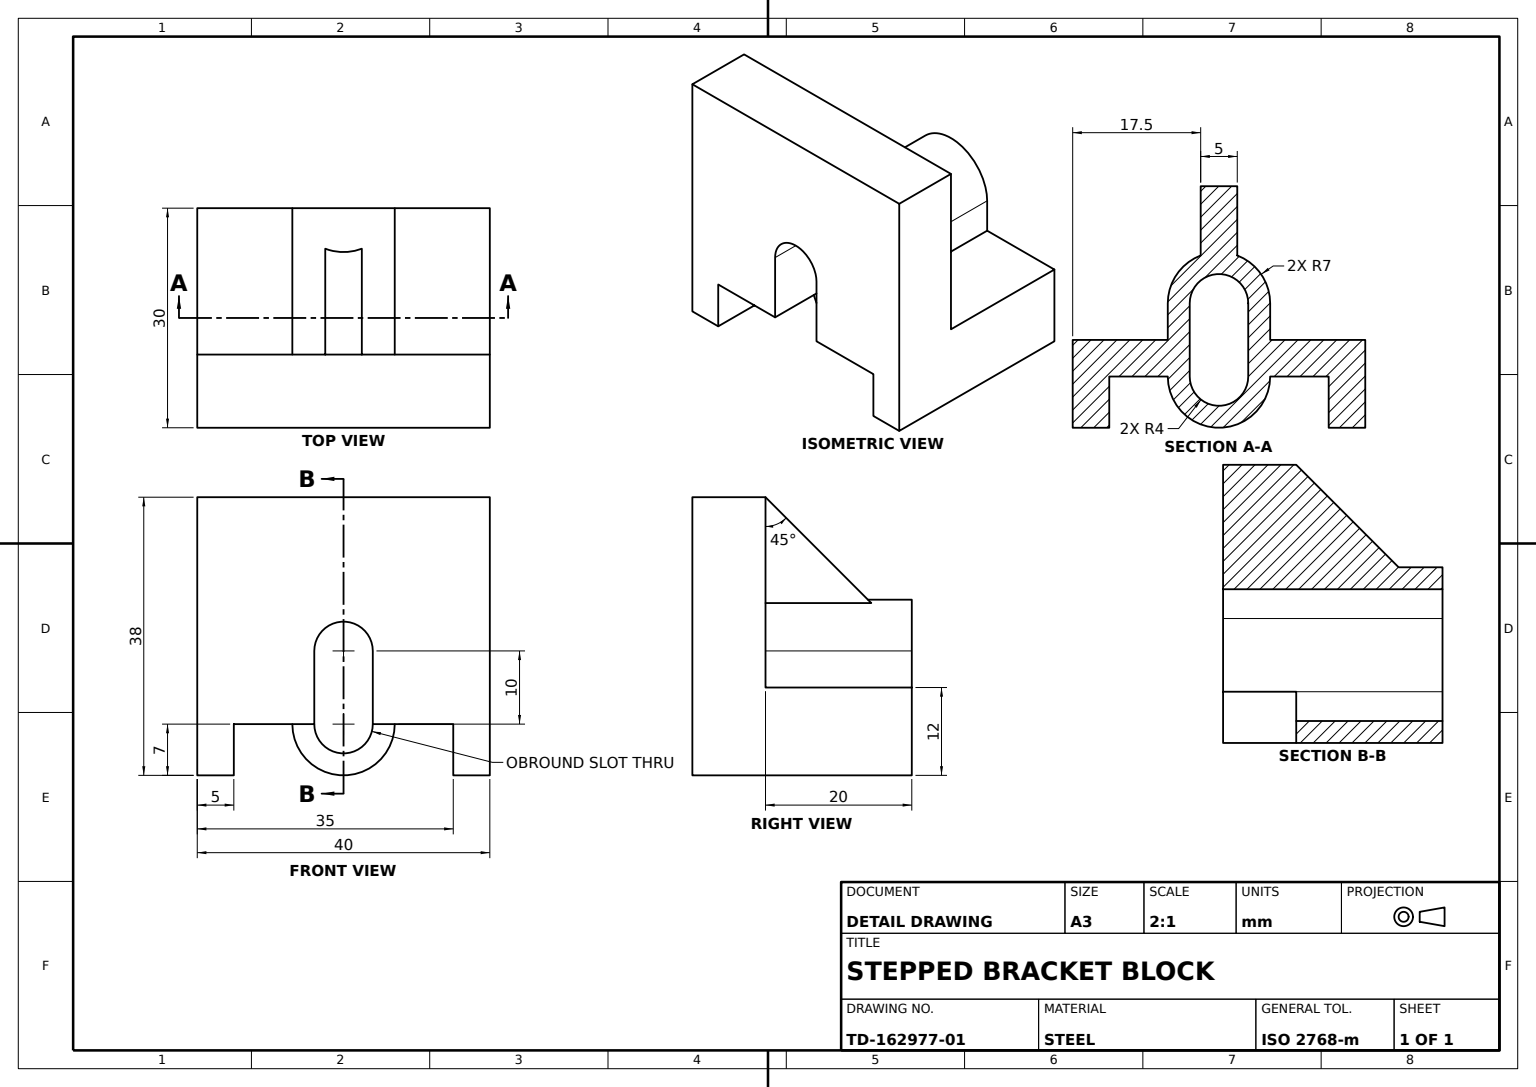
from build123d import *

# Parameters (mm, degrees)
BRACKET_BODY_DEPTH        = 40
BASE_NOTCH_SKETCH_W       = 30
BASE_NOTCH_SKETCH_H       = 7
BASE_NOTCH_CUT_DEPTH      = 63.801273872
CYLINDRICAL_BOSS_DEPTH    = 20
UPRIGHT_OPENING_SKETCH_W  = 8
UPRIGHT_OPENING_SKETCH_H  = 5
UPRIGHT_OPENING_CUT_DEPTH = 20
ARCHED_RELIEF_CUT_DEPTH   = 59.685603004
SUPPORT_RIB_45DEG_REACH   = 54.383
SUPPORT_RIB_SKETCH_WALL_W = 126.565396702
SUPPORT_RIB_SKETCH_WALL_H = 5


with BuildPart() as part:
    # Bracket Profile Sketch → Bracket Body (new body)
    with BuildSketch(Plane.XY):
        Polygon((0, 0), (30, 0), (30, 38), (20, 38), (20, 12), (0, 12), align=None)
    extrude(amount=BRACKET_BODY_DEPTH)

    # Base Notch Sketch → Base Notch Cut (cut, through all)
    with BuildSketch(Plane.ZY):
        with Locations((20, 3.5)):
            Rectangle(BASE_NOTCH_SKETCH_W, BASE_NOTCH_SKETCH_H)
    extrude(amount=-BASE_NOTCH_CUT_DEPTH, mode=Mode.SUBTRACT)

    # Cylindrical Boss Sketch → Cylindrical Boss (add)
    with BuildSketch(Plane.ZY):
        with BuildLine():
            Line((13, 7), (13, 17))
            ThreePointArc((13, 17), (20, 24), (27, 17))
            Line((27, 17), (27, 7))
            ThreePointArc((27, 7), (20, 0), (13, 7))
        make_face()
        with BuildLine():
            Line((16, 7), (16, 17))
            ThreePointArc((16, 17), (20, 21), (24, 17))
            Line((24, 17), (24, 7))
            ThreePointArc((24, 7), (20, 3), (16, 7))
        make_face(mode=Mode.SUBTRACT)
    extrude(amount=-CYLINDRICAL_BOSS_DEPTH)

    # Upright Opening Sketch → Upright Opening Cut (cut)
    with BuildSketch(Plane.ZY):
        with Locations((20, 9.5)):
            Rectangle(UPRIGHT_OPENING_SKETCH_W, UPRIGHT_OPENING_SKETCH_H)
    extrude(amount=-UPRIGHT_OPENING_CUT_DEPTH, mode=Mode.SUBTRACT)

    # Arched Relief Sketch → Arched Relief Cut (cut, through all)
    with BuildSketch(Plane.ZY.offset(-20)):
        with BuildLine():
            Line((16, 17), (16, 7))
            Line((16, 7), (24, 7))
            Line((24, 7), (24, 17))
            ThreePointArc((24, 17), (20, 21), (16, 17))
        make_face()
    extrude(amount=-ARCHED_RELIEF_CUT_DEPTH, mode=Mode.SUBTRACT)

    # Support Rib Sketch wall → Support Rib 45deg (add, up to next)
    with BuildSketch(Plane(origin=(13, 31, 20), x_dir=(-0.707106781187, -0.707106781187, 0), z_dir=(0.707106781187, -0.707106781187, 0)), mode=Mode.PRIVATE) as support_rib_45deg_sk1:
        Rectangle(SUPPORT_RIB_SKETCH_WALL_W, SUPPORT_RIB_SKETCH_WALL_H)
    support_rib_45deg_tool1 = extrude(support_rib_45deg_sk1.sketch, amount=SUPPORT_RIB_45DEG_REACH, mode=Mode.PRIVATE) - part.part
    add(support_rib_45deg_tool1.solids().sort_by_distance((13, 31, 20))[0])


solid = part.part
